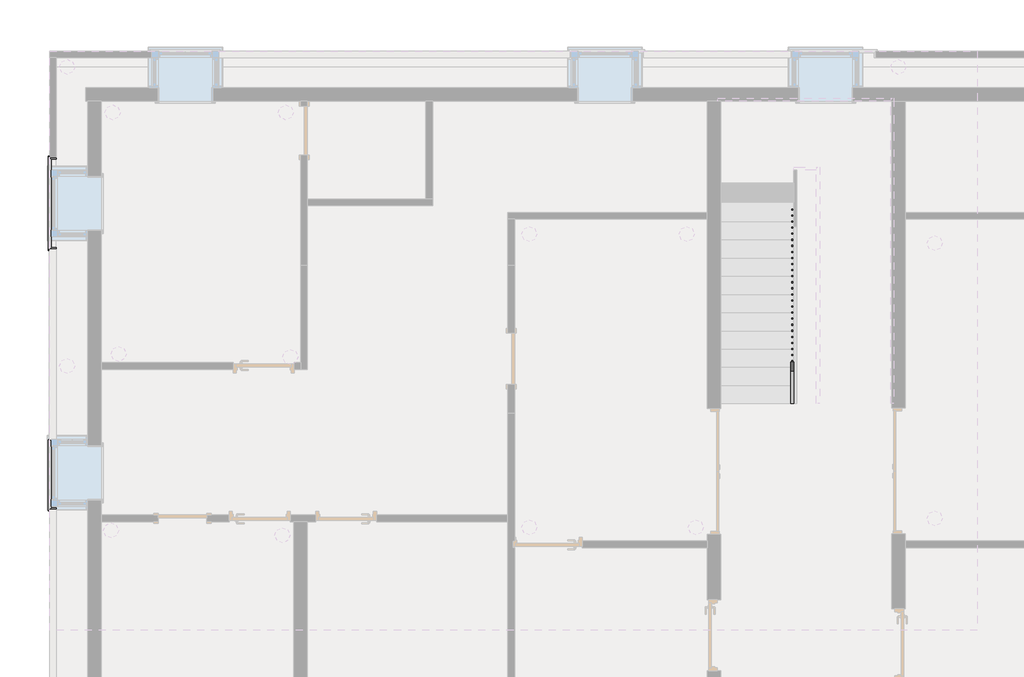
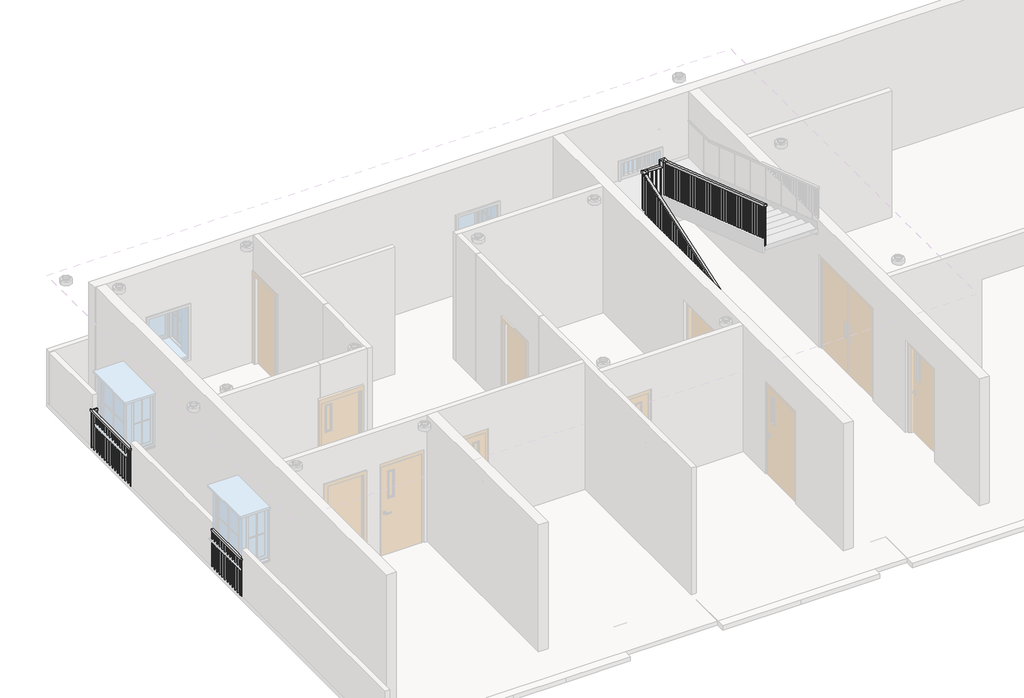
# One storey, part 4 of 7: 3 railings.
"""IFC4 building model written with IfcOpenShell, lengths in millimetres."""

from ifc_helpers import new_model, si_unit, frame, origin, place, context, project, spatial, polyline, outline, extrude, faceted_brep, element, save

model = new_model("IFC4")

# Units and contexts
model_context = context("Model", 3, world=origin())
ifc_project = project(units=[si_unit("LENGTHUNIT", "METRE", prefix="MILLI")], contexts=[model_context])

# Site, building, storey
site = spatial("IfcSite", under=ifc_project)
building = spatial("IfcBuilding", under=site)
storey = spatial("IfcBuildingStorey", under=building, Elevation=3200.4)

# Railings
placement = place(None, origin())
element("IfcRailing", 1, ObjectType="Handrail - Rectangular", at=placement, inside=storey, context=model_context, shape_type="SolidModel", body=[
    faceted_brep([(-680.3987998, 2564.5067329, 4218.2142857), (-680.3987998, 2564.5067329, 4164.5699957), (-629.5987998, 2564.5067329, 4164.5699957), (-629.5987998, 2564.5067329, 4218.2142857), (-680.3987998, 6450.7067329, 5536.7464286), (-680.3987998, 6501.5067329, 5500.3378529), (-629.5987998, 6501.5067329, 5500.3378529), (-629.5987998, 6450.7067329, 5536.7464286), (-553.3987998, 6577.7067329, 5511.8), (-553.3987998, 6577.7067329, 5562.6), (-273.9987915, 6577.7067329, 5562.6), (-223.1987915, 6577.7067329, 5511.8), (-553.3987998, 6526.9067329, 5511.8), (-223.1987915, 6526.9067329, 5511.8), (-553.3987998, 6526.9067329, 5562.6), (-273.9987915, 6526.9067329, 5562.6), (-146.9987915, 2564.5067329, 7010.4), (-197.7987915, 2564.5067329, 7010.4), (-197.7987915, 2564.5067329, 6956.75571), (-146.9987915, 2564.5067329, 6956.75571), (-146.9987915, 6442.3235624, 5641.0678571), (-146.9987915, 6450.7067329, 5691.8678571), (-197.7987915, 6442.3235624, 5641.0678571), (-197.7987915, 6450.7067329, 5691.8678571), (-680.3987998, 6450.7067329, 5562.6), (-680.3987998, 6501.5067329, 5511.8), (-629.5987998, 6501.5067329, 5511.8), (-629.5987998, 6450.7067329, 5562.6), (-680.3987998, 6577.7067329, 5562.6), (-680.3987998, 6577.7067329, 5511.8), (-629.5987998, 6526.9067329, 5511.8), (-629.5987998, 6526.9067329, 5562.6), (-273.9987915, 6577.7067329, 5691.8678571), (-223.1987915, 6577.7067329, 5641.0678571), (-223.1987915, 6526.9067329, 5641.0678571), (-273.9987915, 6526.9067329, 5691.8678571), (-146.9987915, 6577.7067329, 5691.8678571), (-146.9987915, 6577.7067329, 5641.0678571), (-197.7987915, 6526.9067329, 5641.0678571), (-197.7987915, 6526.9067329, 5691.8678571)], [[[0, 1, 2, 3]], [[1, 0, 4, 5]], [[2, 1, 5, 6]], [[3, 2, 6, 7]], [[0, 3, 7, 4]], [[8, 9, 10, 11]], [[12, 8, 11, 13]], [[14, 12, 13, 15]], [[9, 14, 15, 10]], [[16, 17, 18, 19]], [[20, 21, 16, 19]], [[22, 20, 19, 18]], [[23, 22, 18, 17]], [[21, 23, 17, 16]], [[5, 4, 24, 25]], [[6, 5, 25, 26]], [[7, 6, 26, 27]], [[4, 7, 27, 24]], [[25, 24, 28, 29]], [[26, 25, 29, 30]], [[27, 26, 30, 31]], [[24, 27, 31, 28]], [[29, 28, 9, 8]], [[30, 29, 8, 12]], [[31, 30, 12, 14]], [[28, 31, 14, 9]], [[11, 10, 32, 33]], [[13, 11, 33, 34]], [[15, 13, 34, 35]], [[10, 15, 35, 32]], [[33, 32, 36, 37]], [[34, 33, 37, 38]], [[35, 34, 38, 39]], [[32, 35, 39, 36]], [[37, 36, 21, 20]], [[38, 37, 20, 22]], [[39, 38, 22, 23]], [[36, 39, 23, 21]]]),
    extrude(outline(polyline([(2580.3817329, 6951.3695493), (2599.4317329, 6944.9061565), (2599.4317329, 5992.5857143), (2580.3817329, 5992.5857143), (2580.3817329, 6951.3695493)])), frame((-181.9237915, 0.0, 0.0), z_axis=(1.0, 0.0, 0.0), x_axis=(0.0, 1.0, 0.0)), (0.0, 0.0, 1.0), 19.05),
    extrude(outline(polyline([(2681.9817329, 6916.8981207), (2701.0317329, 6910.4347279), (2701.0317329, 5992.5857143), (2681.9817329, 5992.5857143), (2681.9817329, 6916.8981207)])), frame((-181.9237915, 0.0, 0.0), z_axis=(1.0, 0.0, 0.0), x_axis=(0.0, 1.0, 0.0)), (0.0, 0.0, 1.0), 19.05),
    extrude(outline(polyline([(2783.5817329, 6882.4266922), (2802.6317329, 6875.9632993), (2802.6317329, 5992.5857143), (2783.5817329, 5992.5857143), (2783.5817329, 6882.4266922)])), frame((-181.9237915, 0.0, 0.0), z_axis=(1.0, 0.0, 0.0), x_axis=(0.0, 1.0, 0.0)), (0.0, 0.0, 1.0), 19.05),
    extrude(outline(polyline([(2885.1817329, 6847.9552636), (2904.2317329, 6841.4918707), (2904.2317329, 5889.1714286), (2885.1817329, 5889.1714286), (2885.1817329, 6847.9552636)])), frame((-181.9237915, 0.0, 0.0), z_axis=(1.0, 0.0, 0.0), x_axis=(0.0, 1.0, 0.0)), (0.0, 0.0, 1.0), 19.05),
    extrude(outline(polyline([(2986.7817329, 6813.483835), (3005.8317329, 6807.0204422), (3005.8317329, 5889.1714286), (2986.7817329, 5889.1714286), (2986.7817329, 6813.483835)])), frame((-181.9237915, 0.0, 0.0), z_axis=(1.0, 0.0, 0.0), x_axis=(0.0, 1.0, 0.0)), (0.0, 0.0, 1.0), 19.05),
    extrude(outline(polyline([(3088.3817329, 6779.0124065), (3107.4317329, 6772.5490136), (3107.4317329, 5889.1714286), (3088.3817329, 5889.1714286), (3088.3817329, 6779.0124065)])), frame((-181.9237915, 0.0, 0.0), z_axis=(1.0, 0.0, 0.0), x_axis=(0.0, 1.0, 0.0)), (0.0, 0.0, 1.0), 19.05),
    extrude(outline(polyline([(3189.9817329, 6744.5409779), (3209.0317329, 6738.077585), (3209.0317329, 5785.7571429), (3189.9817329, 5785.7571429), (3189.9817329, 6744.5409779)])), frame((-181.9237915, 0.0, 0.0), z_axis=(1.0, 0.0, 0.0), x_axis=(0.0, 1.0, 0.0)), (0.0, 0.0, 1.0), 19.05),
    extrude(outline(polyline([(3291.5817329, 6710.0695493), (3310.6317329, 6703.6061565), (3310.6317329, 5785.7571429), (3291.5817329, 5785.7571429), (3291.5817329, 6710.0695493)])), frame((-181.9237915, 0.0, 0.0), z_axis=(1.0, 0.0, 0.0), x_axis=(0.0, 1.0, 0.0)), (0.0, 0.0, 1.0), 19.05),
    extrude(outline(polyline([(3393.1817329, 6675.5981207), (3412.2317329, 6669.1347279), (3412.2317329, 5785.7571429), (3393.1817329, 5785.7571429), (3393.1817329, 6675.5981207)])), frame((-181.9237915, 0.0, 0.0), z_axis=(1.0, 0.0, 0.0), x_axis=(0.0, 1.0, 0.0)), (0.0, 0.0, 1.0), 19.05),
    extrude(outline(polyline([(3494.7817329, 6641.1266922), (3513.8317329, 6634.6632993), (3513.8317329, 5682.3428571), (3494.7817329, 5682.3428571), (3494.7817329, 6641.1266922)])), frame((-181.9237915, 0.0, 0.0), z_axis=(1.0, 0.0, 0.0), x_axis=(0.0, 1.0, 0.0)), (0.0, 0.0, 1.0), 19.05),
    extrude(outline(polyline([(3596.3817329, 6606.6552636), (3615.4317329, 6600.1918707), (3615.4317329, 5682.3428571), (3596.3817329, 5682.3428571), (3596.3817329, 6606.6552636)])), frame((-181.9237915, 0.0, 0.0), z_axis=(1.0, 0.0, 0.0), x_axis=(0.0, 1.0, 0.0)), (0.0, 0.0, 1.0), 19.05),
    extrude(outline(polyline([(3697.9817329, 6572.183835), (3717.0317329, 6565.7204422), (3717.0317329, 5682.3428571), (3697.9817329, 5682.3428571), (3697.9817329, 6572.183835)])), frame((-181.9237915, 0.0, 0.0), z_axis=(1.0, 0.0, 0.0), x_axis=(0.0, 1.0, 0.0)), (0.0, 0.0, 1.0), 19.05),
    extrude(outline(polyline([(3799.5817329, 6537.7124065), (3818.6317329, 6531.2490136), (3818.6317329, 5578.9285714), (3799.5817329, 5578.9285714), (3799.5817329, 6537.7124065)])), frame((-181.9237915, 0.0, 0.0), z_axis=(1.0, 0.0, 0.0), x_axis=(0.0, 1.0, 0.0)), (0.0, 0.0, 1.0), 19.05),
    extrude(outline(polyline([(3901.1817329, 6503.2409779), (3920.2317329, 6496.777585), (3920.2317329, 5578.9285714), (3901.1817329, 5578.9285714), (3901.1817329, 6503.2409779)])), frame((-181.9237915, 0.0, 0.0), z_axis=(1.0, 0.0, 0.0), x_axis=(0.0, 1.0, 0.0)), (0.0, 0.0, 1.0), 19.05),
    extrude(outline(polyline([(4002.7817329, 6468.7695493), (4021.8317329, 6462.3061565), (4021.8317329, 5578.9285714), (4002.7817329, 5578.9285714), (4002.7817329, 6468.7695493)])), frame((-181.9237915, 0.0, 0.0), z_axis=(1.0, 0.0, 0.0), x_axis=(0.0, 1.0, 0.0)), (0.0, 0.0, 1.0), 19.05),
    extrude(outline(polyline([(4104.3817329, 6434.2981207), (4123.4317329, 6427.8347279), (4123.4317329, 5475.5142857), (4104.3817329, 5475.5142857), (4104.3817329, 6434.2981207)])), frame((-181.9237915, 0.0, 0.0), z_axis=(1.0, 0.0, 0.0), x_axis=(0.0, 1.0, 0.0)), (0.0, 0.0, 1.0), 19.05),
    extrude(outline(polyline([(4205.9817329, 6399.8266922), (4225.0317329, 6393.3632993), (4225.0317329, 5475.5142857), (4205.9817329, 5475.5142857), (4205.9817329, 6399.8266922)])), frame((-181.9237915, 0.0, 0.0), z_axis=(1.0, 0.0, 0.0), x_axis=(0.0, 1.0, 0.0)), (0.0, 0.0, 1.0), 19.05),
    extrude(outline(polyline([(4307.5817329, 6365.3552636), (4326.6317329, 6358.8918707), (4326.6317329, 5475.5142857), (4307.5817329, 5475.5142857), (4307.5817329, 6365.3552636)])), frame((-181.9237915, 0.0, 0.0), z_axis=(1.0, 0.0, 0.0), x_axis=(0.0, 1.0, 0.0)), (0.0, 0.0, 1.0), 19.05),
    extrude(outline(polyline([(4409.1817329, 6330.883835), (4428.2317329, 6324.4204422), (4428.2317329, 5372.1), (4409.1817329, 5372.1), (4409.1817329, 6330.883835)])), frame((-181.9237915, 0.0, 0.0), z_axis=(1.0, 0.0, 0.0), x_axis=(0.0, 1.0, 0.0)), (0.0, 0.0, 1.0), 19.05),
    extrude(outline(polyline([(4510.7817329, 6296.4124065), (4529.8317329, 6289.9490136), (4529.8317329, 5372.1), (4510.7817329, 5372.1), (4510.7817329, 6296.4124065)])), frame((-181.9237915, 0.0, 0.0), z_axis=(1.0, 0.0, 0.0), x_axis=(0.0, 1.0, 0.0)), (0.0, 0.0, 1.0), 19.05),
    extrude(outline(polyline([(4612.3817329, 6261.9409779), (4631.4317329, 6255.477585), (4631.4317329, 5372.1), (4612.3817329, 5372.1), (4612.3817329, 6261.9409779)])), frame((-181.9237915, 0.0, 0.0), z_axis=(1.0, 0.0, 0.0), x_axis=(0.0, 1.0, 0.0)), (0.0, 0.0, 1.0), 19.05),
    extrude(outline(polyline([(4713.9817329, 6227.4695493), (4733.0317329, 6221.0061565), (4733.0317329, 5268.6857143), (4713.9817329, 5268.6857143), (4713.9817329, 6227.4695493)])), frame((-181.9237915, 0.0, 0.0), z_axis=(1.0, 0.0, 0.0), x_axis=(0.0, 1.0, 0.0)), (0.0, 0.0, 1.0), 19.05),
    extrude(outline(polyline([(4815.5817329, 6192.9981207), (4834.6317329, 6186.5347279), (4834.6317329, 5268.6857143), (4815.5817329, 5268.6857143), (4815.5817329, 6192.9981207)])), frame((-181.9237915, 0.0, 0.0), z_axis=(1.0, 0.0, 0.0), x_axis=(0.0, 1.0, 0.0)), (0.0, 0.0, 1.0), 19.05),
    extrude(outline(polyline([(4917.1817329, 6158.5266922), (4936.2317329, 6152.0632993), (4936.2317329, 5268.6857143), (4917.1817329, 5268.6857143), (4917.1817329, 6158.5266922)])), frame((-181.9237915, 0.0, 0.0), z_axis=(1.0, 0.0, 0.0), x_axis=(0.0, 1.0, 0.0)), (0.0, 0.0, 1.0), 19.05),
    extrude(outline(polyline([(5018.7817329, 6124.0552636), (5037.8317329, 6117.5918707), (5037.8317329, 5165.2714286), (5018.7817329, 5165.2714286), (5018.7817329, 6124.0552636)])), frame((-181.9237915, 0.0, 0.0), z_axis=(1.0, 0.0, 0.0), x_axis=(0.0, 1.0, 0.0)), (0.0, 0.0, 1.0), 19.05),
    extrude(outline(polyline([(5120.3817329, 6089.583835), (5139.4317329, 6083.1204422), (5139.4317329, 5165.2714286), (5120.3817329, 5165.2714286), (5120.3817329, 6089.583835)])), frame((-181.9237915, 0.0, 0.0), z_axis=(1.0, 0.0, 0.0), x_axis=(0.0, 1.0, 0.0)), (0.0, 0.0, 1.0), 19.05),
    extrude(outline(polyline([(5221.9817329, 6055.1124065), (5241.0317329, 6048.6490136), (5241.0317329, 5165.2714286), (5221.9817329, 5165.2714286), (5221.9817329, 6055.1124065)])), frame((-181.9237915, 0.0, 0.0), z_axis=(1.0, 0.0, 0.0), x_axis=(0.0, 1.0, 0.0)), (0.0, 0.0, 1.0), 19.05),
    extrude(outline(polyline([(5323.5817329, 6020.6409779), (5342.6317329, 6014.177585), (5342.6317329, 5061.8571429), (5323.5817329, 5061.8571429), (5323.5817329, 6020.6409779)])), frame((-181.9237915, 0.0, 0.0), z_axis=(1.0, 0.0, 0.0), x_axis=(0.0, 1.0, 0.0)), (0.0, 0.0, 1.0), 19.05),
    extrude(outline(polyline([(5425.1817329, 5986.1695493), (5444.2317329, 5979.7061565), (5444.2317329, 5061.8571429), (5425.1817329, 5061.8571429), (5425.1817329, 5986.1695493)])), frame((-181.9237915, 0.0, 0.0), z_axis=(1.0, 0.0, 0.0), x_axis=(0.0, 1.0, 0.0)), (0.0, 0.0, 1.0), 19.05),
    extrude(outline(polyline([(5526.7817329, 5951.6981207), (5545.8317329, 5945.2347279), (5545.8317329, 5061.8571429), (5526.7817329, 5061.8571429), (5526.7817329, 5951.6981207)])), frame((-181.9237915, 0.0, 0.0), z_axis=(1.0, 0.0, 0.0), x_axis=(0.0, 1.0, 0.0)), (0.0, 0.0, 1.0), 19.05),
    extrude(outline(polyline([(5628.3817329, 5917.2266922), (5647.4317329, 5910.7632993), (5647.4317329, 4958.4428571), (5628.3817329, 4958.4428571), (5628.3817329, 5917.2266922)])), frame((-181.9237915, 0.0, 0.0), z_axis=(1.0, 0.0, 0.0), x_axis=(0.0, 1.0, 0.0)), (0.0, 0.0, 1.0), 19.05),
    extrude(outline(polyline([(5729.9817329, 5882.7552636), (5749.0317329, 5876.2918707), (5749.0317329, 4958.4428571), (5729.9817329, 4958.4428571), (5729.9817329, 5882.7552636)])), frame((-181.9237915, 0.0, 0.0), z_axis=(1.0, 0.0, 0.0), x_axis=(0.0, 1.0, 0.0)), (0.0, 0.0, 1.0), 19.05),
    extrude(outline(polyline([(5831.5817329, 5848.283835), (5850.6317329, 5841.8204422), (5850.6317329, 4958.4428571), (5831.5817329, 4958.4428571), (5831.5817329, 5848.283835)])), frame((-181.9237915, 0.0, 0.0), z_axis=(1.0, 0.0, 0.0), x_axis=(0.0, 1.0, 0.0)), (0.0, 0.0, 1.0), 19.05),
    extrude(outline(polyline([(5933.1817329, 5813.8124065), (5952.2317329, 5807.3490136), (5952.2317329, 4855.0285714), (5933.1817329, 4855.0285714), (5933.1817329, 5813.8124065)])), frame((-181.9237915, 0.0, 0.0), z_axis=(1.0, 0.0, 0.0), x_axis=(0.0, 1.0, 0.0)), (0.0, 0.0, 1.0), 19.05),
    extrude(outline(polyline([(6034.7817329, 5779.3409779), (6053.8317329, 5772.877585), (6053.8317329, 4855.0285714), (6034.7817329, 4855.0285714), (6034.7817329, 5779.3409779)])), frame((-181.9237915, 0.0, 0.0), z_axis=(1.0, 0.0, 0.0), x_axis=(0.0, 1.0, 0.0)), (0.0, 0.0, 1.0), 19.05),
    extrude(outline(polyline([(6136.3817329, 5744.8695493), (6155.4317329, 5738.4061565), (6155.4317329, 4855.0285714), (6136.3817329, 4855.0285714), (6136.3817329, 5744.8695493)])), frame((-181.9237915, 0.0, 0.0), z_axis=(1.0, 0.0, 0.0), x_axis=(0.0, 1.0, 0.0)), (0.0, 0.0, 1.0), 19.05),
    extrude(outline(polyline([(6237.9817329, 5710.3981207), (6257.0317329, 5703.9347279), (6257.0317329, 4751.6142857), (6237.9817329, 4751.6142857), (6237.9817329, 5710.3981207)])), frame((-181.9237915, 0.0, 0.0), z_axis=(1.0, 0.0, 0.0), x_axis=(0.0, 1.0, 0.0)), (0.0, 0.0, 1.0), 19.05),
    extrude(outline(polyline([(6339.5817329, 5675.9266922), (6358.6317329, 5669.4632993), (6358.6317329, 4751.6142857), (6339.5817329, 4751.6142857), (6339.5817329, 5675.9266922)])), frame((-181.9237915, 0.0, 0.0), z_axis=(1.0, 0.0, 0.0), x_axis=(0.0, 1.0, 0.0)), (0.0, 0.0, 1.0), 19.05),
    extrude(outline(polyline([(6441.1817329, 5641.4552636), (6460.2317329, 5634.9918707), (6460.2317329, 4751.6142857), (6441.1817329, 4751.6142857), (6441.1817329, 5641.4552636)])), frame((-181.9237915, 0.0, 0.0), z_axis=(1.0, 0.0, 0.0), x_axis=(0.0, 1.0, 0.0)), (0.0, 0.0, 1.0), 19.05),
    extrude(outline(polyline([(-258.1237998, 6542.7817329), (-258.1237998, 6561.8317329), (-239.0737998, 6561.8317329), (-239.0737998, 6542.7817329), (-258.1237998, 6542.7817329)])), frame((0.0, 0.0, 4648.2), z_axis=(0.0, 0.0, 1.0), x_axis=(1.0, 0.0, 0.0)), (0.0, 0.0, 1.0), 992.8678571),
    extrude(outline(polyline([(-359.7237998, 6542.7817329), (-359.7237998, 6561.8317329), (-340.6737998, 6561.8317329), (-340.6737998, 6542.7817329), (-359.7237998, 6542.7817329)])), frame((0.0, 0.0, 4648.2), z_axis=(0.0, 0.0, 1.0), x_axis=(1.0, 0.0, 0.0)), (0.0, 0.0, 1.0), 863.6),
    extrude(outline(polyline([(-461.3237998, 6542.7817329), (-461.3237998, 6561.8317329), (-442.2737998, 6561.8317329), (-442.2737998, 6542.7817329), (-461.3237998, 6542.7817329)])), frame((0.0, 0.0, 4648.2), z_axis=(0.0, 0.0, 1.0), x_axis=(1.0, 0.0, 0.0)), (0.0, 0.0, 1.0), 863.6),
    extrude(outline(polyline([(-562.9237998, 6542.7817329), (-562.9237998, 6561.8317329), (-543.8737998, 6561.8317329), (-543.8737998, 6542.7817329), (-562.9237998, 6542.7817329)])), frame((0.0, 0.0, 4648.2), z_axis=(0.0, 0.0, 1.0), x_axis=(1.0, 0.0, 0.0)), (0.0, 0.0, 1.0), 863.6),
    extrude(outline(polyline([(-645.4737998, 6517.3817329), (-664.5237998, 6517.3817329), (-664.5237998, 6536.4317329), (-645.4737998, 6536.4317329), (-645.4737998, 6517.3817329)])), frame((0.0, 0.0, 4648.2), z_axis=(0.0, 0.0, 1.0), x_axis=(1.0, 0.0, 0.0)), (0.0, 0.0, 1.0), 863.6),
    extrude(outline(polyline([(6415.7817329, 5471.252585), (6434.8317329, 5477.7159779), (6434.8317329, 4544.7857143), (6415.7817329, 4544.7857143), (6415.7817329, 5471.252585)])), frame((-664.5237998, 0.0, 0.0), z_axis=(1.0, 0.0, 0.0), x_axis=(0.0, 1.0, 0.0)), (0.0, 0.0, 1.0), 19.05),
    extrude(outline(polyline([(6314.1817329, 5436.7811565), (6333.2317329, 5443.2445493), (6333.2317329, 4544.7857143), (6314.1817329, 4544.7857143), (6314.1817329, 5436.7811565)])), frame((-664.5237998, 0.0, 0.0), z_axis=(1.0, 0.0, 0.0), x_axis=(0.0, 1.0, 0.0)), (0.0, 0.0, 1.0), 19.05),
    extrude(outline(polyline([(6212.5817329, 5402.3097279), (6231.6317329, 5408.7731207), (6231.6317329, 4544.7857143), (6212.5817329, 4544.7857143), (6212.5817329, 5402.3097279)])), frame((-664.5237998, 0.0, 0.0), z_axis=(1.0, 0.0, 0.0), x_axis=(0.0, 1.0, 0.0)), (0.0, 0.0, 1.0), 19.05),
    extrude(outline(polyline([(6110.9817329, 5367.8382993), (6130.0317329, 5374.3016922), (6130.0317329, 4441.3714286), (6110.9817329, 4441.3714286), (6110.9817329, 5367.8382993)])), frame((-664.5237998, 0.0, 0.0), z_axis=(1.0, 0.0, 0.0), x_axis=(0.0, 1.0, 0.0)), (0.0, 0.0, 1.0), 19.05),
    extrude(outline(polyline([(6009.3817329, 5333.3668707), (6028.4317329, 5339.8302636), (6028.4317329, 4441.3714286), (6009.3817329, 4441.3714286), (6009.3817329, 5333.3668707)])), frame((-664.5237998, 0.0, 0.0), z_axis=(1.0, 0.0, 0.0), x_axis=(0.0, 1.0, 0.0)), (0.0, 0.0, 1.0), 19.05),
    extrude(outline(polyline([(5907.7817329, 5298.8954422), (5926.8317329, 5305.358835), (5926.8317329, 4441.3714286), (5907.7817329, 4441.3714286), (5907.7817329, 5298.8954422)])), frame((-664.5237998, 0.0, 0.0), z_axis=(1.0, 0.0, 0.0), x_axis=(0.0, 1.0, 0.0)), (0.0, 0.0, 1.0), 19.05),
    extrude(outline(polyline([(5806.1817329, 5264.4240136), (5825.2317329, 5270.8874065), (5825.2317329, 4337.9571429), (5806.1817329, 4337.9571429), (5806.1817329, 5264.4240136)])), frame((-664.5237998, 0.0, 0.0), z_axis=(1.0, 0.0, 0.0), x_axis=(0.0, 1.0, 0.0)), (0.0, 0.0, 1.0), 19.05),
    extrude(outline(polyline([(5704.5817329, 5229.952585), (5723.6317329, 5236.4159779), (5723.6317329, 4337.9571429), (5704.5817329, 4337.9571429), (5704.5817329, 5229.952585)])), frame((-664.5237998, 0.0, 0.0), z_axis=(1.0, 0.0, 0.0), x_axis=(0.0, 1.0, 0.0)), (0.0, 0.0, 1.0), 19.05),
    extrude(outline(polyline([(5602.9817329, 5195.4811565), (5622.0317329, 5201.9445493), (5622.0317329, 4337.9571429), (5602.9817329, 4337.9571429), (5602.9817329, 5195.4811565)])), frame((-664.5237998, 0.0, 0.0), z_axis=(1.0, 0.0, 0.0), x_axis=(0.0, 1.0, 0.0)), (0.0, 0.0, 1.0), 19.05),
    extrude(outline(polyline([(5501.3817329, 5161.0097279), (5520.4317329, 5167.4731207), (5520.4317329, 4234.5428571), (5501.3817329, 4234.5428571), (5501.3817329, 5161.0097279)])), frame((-664.5237998, 0.0, 0.0), z_axis=(1.0, 0.0, 0.0), x_axis=(0.0, 1.0, 0.0)), (0.0, 0.0, 1.0), 19.05),
    extrude(outline(polyline([(5399.7817329, 5126.5382993), (5418.8317329, 5133.0016922), (5418.8317329, 4234.5428571), (5399.7817329, 4234.5428571), (5399.7817329, 5126.5382993)])), frame((-664.5237998, 0.0, 0.0), z_axis=(1.0, 0.0, 0.0), x_axis=(0.0, 1.0, 0.0)), (0.0, 0.0, 1.0), 19.05),
    extrude(outline(polyline([(5298.1817329, 5092.0668707), (5317.2317329, 5098.5302636), (5317.2317329, 4234.5428571), (5298.1817329, 4234.5428571), (5298.1817329, 5092.0668707)])), frame((-664.5237998, 0.0, 0.0), z_axis=(1.0, 0.0, 0.0), x_axis=(0.0, 1.0, 0.0)), (0.0, 0.0, 1.0), 19.05),
    extrude(outline(polyline([(5196.5817329, 5057.5954422), (5215.6317329, 5064.058835), (5215.6317329, 4131.1285714), (5196.5817329, 4131.1285714), (5196.5817329, 5057.5954422)])), frame((-664.5237998, 0.0, 0.0), z_axis=(1.0, 0.0, 0.0), x_axis=(0.0, 1.0, 0.0)), (0.0, 0.0, 1.0), 19.05),
    extrude(outline(polyline([(5094.9817329, 5023.1240136), (5114.0317329, 5029.5874065), (5114.0317329, 4131.1285714), (5094.9817329, 4131.1285714), (5094.9817329, 5023.1240136)])), frame((-664.5237998, 0.0, 0.0), z_axis=(1.0, 0.0, 0.0), x_axis=(0.0, 1.0, 0.0)), (0.0, 0.0, 1.0), 19.05),
    extrude(outline(polyline([(4993.3817329, 4988.652585), (5012.4317329, 4995.1159779), (5012.4317329, 4131.1285714), (4993.3817329, 4131.1285714), (4993.3817329, 4988.652585)])), frame((-664.5237998, 0.0, 0.0), z_axis=(1.0, 0.0, 0.0), x_axis=(0.0, 1.0, 0.0)), (0.0, 0.0, 1.0), 19.05),
    extrude(outline(polyline([(4891.7817329, 4954.1811565), (4910.8317329, 4960.6445493), (4910.8317329, 4027.7142857), (4891.7817329, 4027.7142857), (4891.7817329, 4954.1811565)])), frame((-664.5237998, 0.0, 0.0), z_axis=(1.0, 0.0, 0.0), x_axis=(0.0, 1.0, 0.0)), (0.0, 0.0, 1.0), 19.05),
    extrude(outline(polyline([(4790.1817329, 4919.7097279), (4809.2317329, 4926.1731207), (4809.2317329, 4027.7142857), (4790.1817329, 4027.7142857), (4790.1817329, 4919.7097279)])), frame((-664.5237998, 0.0, 0.0), z_axis=(1.0, 0.0, 0.0), x_axis=(0.0, 1.0, 0.0)), (0.0, 0.0, 1.0), 19.05),
    extrude(outline(polyline([(4688.5817329, 4885.2382993), (4707.6317329, 4891.7016922), (4707.6317329, 4027.7142857), (4688.5817329, 4027.7142857), (4688.5817329, 4885.2382993)])), frame((-664.5237998, 0.0, 0.0), z_axis=(1.0, 0.0, 0.0), x_axis=(0.0, 1.0, 0.0)), (0.0, 0.0, 1.0), 19.05),
    extrude(outline(polyline([(4586.9817329, 4850.7668707), (4606.0317329, 4857.2302636), (4606.0317329, 3924.3), (4586.9817329, 3924.3), (4586.9817329, 4850.7668707)])), frame((-664.5237998, 0.0, 0.0), z_axis=(1.0, 0.0, 0.0), x_axis=(0.0, 1.0, 0.0)), (0.0, 0.0, 1.0), 19.05),
    extrude(outline(polyline([(4485.3817329, 4816.2954422), (4504.4317329, 4822.758835), (4504.4317329, 3924.3), (4485.3817329, 3924.3), (4485.3817329, 4816.2954422)])), frame((-664.5237998, 0.0, 0.0), z_axis=(1.0, 0.0, 0.0), x_axis=(0.0, 1.0, 0.0)), (0.0, 0.0, 1.0), 19.05),
    extrude(outline(polyline([(4383.7817329, 4781.8240136), (4402.8317329, 4788.2874065), (4402.8317329, 3924.3), (4383.7817329, 3924.3), (4383.7817329, 4781.8240136)])), frame((-664.5237998, 0.0, 0.0), z_axis=(1.0, 0.0, 0.0), x_axis=(0.0, 1.0, 0.0)), (0.0, 0.0, 1.0), 19.05),
    extrude(outline(polyline([(4282.1817329, 4747.352585), (4301.2317329, 4753.8159779), (4301.2317329, 3820.8857143), (4282.1817329, 3820.8857143), (4282.1817329, 4747.352585)])), frame((-664.5237998, 0.0, 0.0), z_axis=(1.0, 0.0, 0.0), x_axis=(0.0, 1.0, 0.0)), (0.0, 0.0, 1.0), 19.05),
    extrude(outline(polyline([(4180.5817329, 4712.8811565), (4199.6317329, 4719.3445493), (4199.6317329, 3820.8857143), (4180.5817329, 3820.8857143), (4180.5817329, 4712.8811565)])), frame((-664.5237998, 0.0, 0.0), z_axis=(1.0, 0.0, 0.0), x_axis=(0.0, 1.0, 0.0)), (0.0, 0.0, 1.0), 19.05),
    extrude(outline(polyline([(4078.9817329, 4678.4097279), (4098.0317329, 4684.8731207), (4098.0317329, 3820.8857143), (4078.9817329, 3820.8857143), (4078.9817329, 4678.4097279)])), frame((-664.5237998, 0.0, 0.0), z_axis=(1.0, 0.0, 0.0), x_axis=(0.0, 1.0, 0.0)), (0.0, 0.0, 1.0), 19.05),
    extrude(outline(polyline([(3977.3817329, 4643.9382993), (3996.4317329, 4650.4016922), (3996.4317329, 3717.4714286), (3977.3817329, 3717.4714286), (3977.3817329, 4643.9382993)])), frame((-664.5237998, 0.0, 0.0), z_axis=(1.0, 0.0, 0.0), x_axis=(0.0, 1.0, 0.0)), (0.0, 0.0, 1.0), 19.05),
    extrude(outline(polyline([(3875.7817329, 4609.4668707), (3894.8317329, 4615.9302636), (3894.8317329, 3717.4714286), (3875.7817329, 3717.4714286), (3875.7817329, 4609.4668707)])), frame((-664.5237998, 0.0, 0.0), z_axis=(1.0, 0.0, 0.0), x_axis=(0.0, 1.0, 0.0)), (0.0, 0.0, 1.0), 19.05),
    extrude(outline(polyline([(3774.1817329, 4574.9954422), (3793.2317329, 4581.458835), (3793.2317329, 3717.4714286), (3774.1817329, 3717.4714286), (3774.1817329, 4574.9954422)])), frame((-664.5237998, 0.0, 0.0), z_axis=(1.0, 0.0, 0.0), x_axis=(0.0, 1.0, 0.0)), (0.0, 0.0, 1.0), 19.05),
    extrude(outline(polyline([(3672.5817329, 4540.5240136), (3691.6317329, 4546.9874065), (3691.6317329, 3614.0571429), (3672.5817329, 3614.0571429), (3672.5817329, 4540.5240136)])), frame((-664.5237998, 0.0, 0.0), z_axis=(1.0, 0.0, 0.0), x_axis=(0.0, 1.0, 0.0)), (0.0, 0.0, 1.0), 19.05),
    extrude(outline(polyline([(3570.9817329, 4506.052585), (3590.0317329, 4512.5159779), (3590.0317329, 3614.0571429), (3570.9817329, 3614.0571429), (3570.9817329, 4506.052585)])), frame((-664.5237998, 0.0, 0.0), z_axis=(1.0, 0.0, 0.0), x_axis=(0.0, 1.0, 0.0)), (0.0, 0.0, 1.0), 19.05),
    extrude(outline(polyline([(3469.3817329, 4471.5811565), (3488.4317329, 4478.0445493), (3488.4317329, 3614.0571429), (3469.3817329, 3614.0571429), (3469.3817329, 4471.5811565)])), frame((-664.5237998, 0.0, 0.0), z_axis=(1.0, 0.0, 0.0), x_axis=(0.0, 1.0, 0.0)), (0.0, 0.0, 1.0), 19.05),
    extrude(outline(polyline([(3367.7817329, 4437.1097279), (3386.8317329, 4443.5731207), (3386.8317329, 3510.6428571), (3367.7817329, 3510.6428571), (3367.7817329, 4437.1097279)])), frame((-664.5237998, 0.0, 0.0), z_axis=(1.0, 0.0, 0.0), x_axis=(0.0, 1.0, 0.0)), (0.0, 0.0, 1.0), 19.05),
    extrude(outline(polyline([(3266.1817329, 4402.6382993), (3285.2317329, 4409.1016922), (3285.2317329, 3510.6428571), (3266.1817329, 3510.6428571), (3266.1817329, 4402.6382993)])), frame((-664.5237998, 0.0, 0.0), z_axis=(1.0, 0.0, 0.0), x_axis=(0.0, 1.0, 0.0)), (0.0, 0.0, 1.0), 19.05),
    extrude(outline(polyline([(3164.5817329, 4368.1668707), (3183.6317329, 4374.6302636), (3183.6317329, 3510.6428571), (3164.5817329, 3510.6428571), (3164.5817329, 4368.1668707)])), frame((-664.5237998, 0.0, 0.0), z_axis=(1.0, 0.0, 0.0), x_axis=(0.0, 1.0, 0.0)), (0.0, 0.0, 1.0), 19.05),
    extrude(outline(polyline([(3062.9817329, 4333.6954422), (3082.0317329, 4340.158835), (3082.0317329, 3407.2285714), (3062.9817329, 3407.2285714), (3062.9817329, 4333.6954422)])), frame((-664.5237998, 0.0, 0.0), z_axis=(1.0, 0.0, 0.0), x_axis=(0.0, 1.0, 0.0)), (0.0, 0.0, 1.0), 19.05),
    extrude(outline(polyline([(2961.3817329, 4299.2240136), (2980.4317329, 4305.6874065), (2980.4317329, 3407.2285714), (2961.3817329, 3407.2285714), (2961.3817329, 4299.2240136)])), frame((-664.5237998, 0.0, 0.0), z_axis=(1.0, 0.0, 0.0), x_axis=(0.0, 1.0, 0.0)), (0.0, 0.0, 1.0), 19.05),
    extrude(outline(polyline([(2859.7817329, 4264.752585), (2878.8317329, 4271.2159779), (2878.8317329, 3407.2285714), (2859.7817329, 3407.2285714), (2859.7817329, 4264.752585)])), frame((-664.5237998, 0.0, 0.0), z_axis=(1.0, 0.0, 0.0), x_axis=(0.0, 1.0, 0.0)), (0.0, 0.0, 1.0), 19.05),
    extrude(outline(polyline([(2758.1817329, 4230.2811565), (2777.2317329, 4236.7445493), (2777.2317329, 3303.8142857), (2758.1817329, 3303.8142857), (2758.1817329, 4230.2811565)])), frame((-664.5237998, 0.0, 0.0), z_axis=(1.0, 0.0, 0.0), x_axis=(0.0, 1.0, 0.0)), (0.0, 0.0, 1.0), 19.05),
    extrude(outline(polyline([(2656.5817329, 4195.8097279), (2675.6317329, 4202.2731207), (2675.6317329, 3303.8142857), (2656.5817329, 3303.8142857), (2656.5817329, 4195.8097279)])), frame((-664.5237998, 0.0, 0.0), z_axis=(1.0, 0.0, 0.0), x_axis=(0.0, 1.0, 0.0)), (0.0, 0.0, 1.0), 19.05),
    extrude(outline(polyline([(-181.9237915, 6542.7817329), (-181.9237915, 6561.8317329), (-162.8737915, 6561.8317329), (-162.8737915, 6542.7817329), (-181.9237915, 6542.7817329)])), frame((0.0, 0.0, 4648.2), z_axis=(0.0, 0.0, 1.0), x_axis=(1.0, 0.0, 0.0)), (0.0, 0.0, 1.0), 992.8678571),
    extrude(outline(polyline([(-645.4737998, 6542.7817329), (-664.5237998, 6542.7817329), (-664.5237998, 6561.8317329), (-645.4737998, 6561.8317329), (-645.4737998, 6542.7817329)])), frame((0.0, 0.0, 4648.2), z_axis=(0.0, 0.0, 1.0), x_axis=(1.0, 0.0, 0.0)), (0.0, 0.0, 1.0), 863.6),
    extrude(outline(polyline([(2564.5067329, 6956.75571), (2583.5567329, 6950.2923172), (2583.5567329, 5992.5857143), (2564.5067329, 5992.5857143), (2564.5067329, 6956.75571)])), frame((-181.9237915, 0.0, 0.0), z_axis=(1.0, 0.0, 0.0), x_axis=(0.0, 1.0, 0.0)), (0.0, 0.0, 1.0), 19.05),
    extrude(outline(polyline([(2564.5067329, 4164.5699957), (2583.5567329, 4171.0333886), (2583.5567329, 3303.8142857), (2564.5067329, 3303.8142857), (2564.5067329, 4164.5699957)])), frame((-664.5237998, 0.0, 0.0), z_axis=(1.0, 0.0, 0.0), x_axis=(0.0, 1.0, 0.0)), (0.0, 0.0, 1.0), 19.05),
])
element("IfcRailing", 2, ObjectType="Handrail - Rectangular", at=placement, inside=storey, context=model_context, shape_type="SolidModel", body=[
    faceted_brep([(-13063.4067989, 1953.9604213, 4114.8), (-13063.4067989, 1953.9604213, 4064.0), (-13114.2067989, 1953.9604213, 4064.0), (-13114.2067989, 1953.9604213, 4114.8), (-13063.4067989, 818.2567339, 4114.8), (-13063.4067989, 818.2567339, 4064.0), (-13114.2067989, 767.4567339, 4064.0), (-13114.2067989, 767.4567339, 4114.8), (-12974.5067989, 818.2567339, 4114.8), (-12974.5067989, 767.4567339, 4114.8), (-12974.5067989, 767.4567339, 4064.0), (-12974.5067989, 818.2567339, 4064.0)], [[[0, 1, 2, 3]], [[1, 0, 4, 5]], [[2, 1, 5, 6]], [[3, 2, 6, 7]], [[0, 3, 7, 4]], [[8, 9, 10, 11]], [[5, 4, 8, 11]], [[6, 5, 11, 10]], [[7, 6, 10, 9]], [[4, 7, 9, 8]]]),
    extrude(outline(polyline([(-12996.7317989, 783.3317339), (-12996.7317989, 802.3817339), (-12977.6817989, 802.3817339), (-12977.6817989, 783.3317339), (-12996.7317989, 783.3317339)])), frame((0.0, 0.0, 3200.4), z_axis=(0.0, 0.0, 1.0), x_axis=(1.0, 0.0, 0.0)), (0.0, 0.0, 1.0), 863.6),
    extrude(outline(polyline([(-13098.3317989, 845.8854213), (-13079.2817989, 845.8854213), (-13079.2817989, 826.8354213), (-13098.3317989, 826.8354213), (-13098.3317989, 845.8854213)])), frame((0.0, 0.0, 3200.4), z_axis=(0.0, 0.0, 1.0), x_axis=(1.0, 0.0, 0.0)), (0.0, 0.0, 1.0), 863.6),
    extrude(outline(polyline([(-13098.3317989, 947.4854213), (-13079.2817989, 947.4854213), (-13079.2817989, 928.4354213), (-13098.3317989, 928.4354213), (-13098.3317989, 947.4854213)])), frame((0.0, 0.0, 3200.4), z_axis=(0.0, 0.0, 1.0), x_axis=(1.0, 0.0, 0.0)), (0.0, 0.0, 1.0), 863.6),
    extrude(outline(polyline([(-13098.3317989, 1049.0854213), (-13079.2817989, 1049.0854213), (-13079.2817989, 1030.0354213), (-13098.3317989, 1030.0354213), (-13098.3317989, 1049.0854213)])), frame((0.0, 0.0, 3200.4), z_axis=(0.0, 0.0, 1.0), x_axis=(1.0, 0.0, 0.0)), (0.0, 0.0, 1.0), 863.6),
    extrude(outline(polyline([(-13098.3317989, 1150.6854213), (-13079.2817989, 1150.6854213), (-13079.2817989, 1131.6354213), (-13098.3317989, 1131.6354213), (-13098.3317989, 1150.6854213)])), frame((0.0, 0.0, 3200.4), z_axis=(0.0, 0.0, 1.0), x_axis=(1.0, 0.0, 0.0)), (0.0, 0.0, 1.0), 863.6),
    extrude(outline(polyline([(-13098.3317989, 1252.2854213), (-13079.2817989, 1252.2854213), (-13079.2817989, 1233.2354213), (-13098.3317989, 1233.2354213), (-13098.3317989, 1252.2854213)])), frame((0.0, 0.0, 3200.4), z_axis=(0.0, 0.0, 1.0), x_axis=(1.0, 0.0, 0.0)), (0.0, 0.0, 1.0), 863.6),
    extrude(outline(polyline([(-13098.3317989, 1353.8854213), (-13079.2817989, 1353.8854213), (-13079.2817989, 1334.8354213), (-13098.3317989, 1334.8354213), (-13098.3317989, 1353.8854213)])), frame((0.0, 0.0, 3200.4), z_axis=(0.0, 0.0, 1.0), x_axis=(1.0, 0.0, 0.0)), (0.0, 0.0, 1.0), 863.6),
    extrude(outline(polyline([(-13098.3317989, 1455.4854213), (-13079.2817989, 1455.4854213), (-13079.2817989, 1436.4354213), (-13098.3317989, 1436.4354213), (-13098.3317989, 1455.4854213)])), frame((0.0, 0.0, 3200.4), z_axis=(0.0, 0.0, 1.0), x_axis=(1.0, 0.0, 0.0)), (0.0, 0.0, 1.0), 863.6),
    extrude(outline(polyline([(-13098.3317989, 1557.0854213), (-13079.2817989, 1557.0854213), (-13079.2817989, 1538.0354213), (-13098.3317989, 1538.0354213), (-13098.3317989, 1557.0854213)])), frame((0.0, 0.0, 3200.4), z_axis=(0.0, 0.0, 1.0), x_axis=(1.0, 0.0, 0.0)), (0.0, 0.0, 1.0), 863.6),
    extrude(outline(polyline([(-13098.3317989, 1658.6854213), (-13079.2817989, 1658.6854213), (-13079.2817989, 1639.6354213), (-13098.3317989, 1639.6354213), (-13098.3317989, 1658.6854213)])), frame((0.0, 0.0, 3200.4), z_axis=(0.0, 0.0, 1.0), x_axis=(1.0, 0.0, 0.0)), (0.0, 0.0, 1.0), 863.6),
    extrude(outline(polyline([(-13098.3317989, 1760.2854213), (-13079.2817989, 1760.2854213), (-13079.2817989, 1741.2354213), (-13098.3317989, 1741.2354213), (-13098.3317989, 1760.2854213)])), frame((0.0, 0.0, 3200.4), z_axis=(0.0, 0.0, 1.0), x_axis=(1.0, 0.0, 0.0)), (0.0, 0.0, 1.0), 863.6),
    extrude(outline(polyline([(-13098.3317989, 1861.8854213), (-13079.2817989, 1861.8854213), (-13079.2817989, 1842.8354213), (-13098.3317989, 1842.8354213), (-13098.3317989, 1861.8854213)])), frame((0.0, 0.0, 3200.4), z_axis=(0.0, 0.0, 1.0), x_axis=(1.0, 0.0, 0.0)), (0.0, 0.0, 1.0), 863.6),
    extrude(outline(polyline([(-13098.3317989, 802.3817339), (-13079.2817989, 802.3817339), (-13079.2817989, 783.3317339), (-13098.3317989, 783.3317339), (-13098.3317989, 802.3817339)])), frame((0.0, 0.0, 3200.4), z_axis=(0.0, 0.0, 1.0), x_axis=(1.0, 0.0, 0.0)), (0.0, 0.0, 1.0), 863.6),
    extrude(outline(polyline([(-13079.2817989, 1963.4854213), (-13079.2817989, 1944.4354213), (-13098.3317989, 1944.4354213), (-13098.3317989, 1963.4854213), (-13079.2817989, 1963.4854213)])), frame((0.0, 0.0, 3200.4), z_axis=(0.0, 0.0, 1.0), x_axis=(1.0, 0.0, 0.0)), (0.0, 0.0, 1.0), 863.6),
    extrude(outline(polyline([(-12993.5567989, 783.3317339), (-12993.5567989, 802.3817339), (-12974.5067989, 802.3817339), (-12974.5067989, 783.3317339), (-12993.5567989, 783.3317339)])), frame((0.0, 0.0, 3200.4), z_axis=(0.0, 0.0, 1.0), x_axis=(1.0, 0.0, 0.0)), (0.0, 0.0, 1.0), 863.6),
    extrude(outline(polyline([(-13062.8987925, 1963.4854213), (-13062.8987925, 1944.4354213), (-13081.9487925, 1944.4354213), (-13081.9487925, 1963.4854213), (-13062.8987925, 1963.4854213)])), frame((0.0, 0.0, 3200.4), z_axis=(0.0, 0.0, 1.0), x_axis=(1.0, 0.0, 0.0)), (0.0, 0.0, 1.0), 863.6),
])
element("IfcRailing", 3, ObjectType="Handrail - Rectangular", at=placement, inside=storey, context=model_context, shape_type="SolidModel", body=[
    faceted_brep([(-12973.9987925, 6656.8711337, 4114.8), (-12973.9987925, 6656.8711337, 4064.0), (-12973.9987925, 6707.6711337, 4064.0), (-12973.9987925, 6707.6711337, 4114.8), (-13062.8987925, 6656.8711337, 4114.8), (-13062.8987925, 6656.8711337, 4064.0), (-13113.6987925, 6707.6711337, 4064.0), (-13113.6987925, 6707.6711337, 4114.8), (-13062.8987925, 5180.1736362, 4114.8), (-13062.8987925, 5180.1736362, 4064.0), (-13113.6987925, 5129.3736362, 4064.0), (-13113.6987925, 5129.3736362, 4114.8), (-12973.9987925, 5180.1736362, 4114.8), (-12973.9987925, 5129.3736362, 4114.8), (-12973.9987925, 5129.3736362, 4064.0), (-12973.9987925, 5180.1736362, 4064.0)], [[[0, 1, 2, 3]], [[1, 0, 4, 5]], [[2, 1, 5, 6]], [[3, 2, 6, 7]], [[0, 3, 7, 4]], [[5, 4, 8, 9]], [[6, 5, 9, 10]], [[7, 6, 10, 11]], [[4, 7, 11, 8]], [[12, 13, 14, 15]], [[9, 8, 12, 15]], [[10, 9, 15, 14]], [[11, 10, 14, 13]], [[8, 11, 13, 12]]]),
    extrude(outline(polyline([(-12996.2237925, 5145.2486362), (-12996.2237925, 5164.2986362), (-12977.1737925, 5164.2986362), (-12977.1737925, 5145.2486362), (-12996.2237925, 5145.2486362)])), frame((0.0, 0.0, 3200.4), z_axis=(0.0, 0.0, 1.0), x_axis=(1.0, 0.0, 0.0)), (0.0, 0.0, 1.0), 863.6),
    extrude(outline(polyline([(-13097.8237925, 5167.7961337), (-13078.7737925, 5167.7961337), (-13078.7737925, 5148.7461337), (-13097.8237925, 5148.7461337), (-13097.8237925, 5167.7961337)])), frame((0.0, 0.0, 3200.4), z_axis=(0.0, 0.0, 1.0), x_axis=(1.0, 0.0, 0.0)), (0.0, 0.0, 1.0), 863.6),
    extrude(outline(polyline([(-13097.8237925, 5269.3961337), (-13078.7737925, 5269.3961337), (-13078.7737925, 5250.3461337), (-13097.8237925, 5250.3461337), (-13097.8237925, 5269.3961337)])), frame((0.0, 0.0, 3200.4), z_axis=(0.0, 0.0, 1.0), x_axis=(1.0, 0.0, 0.0)), (0.0, 0.0, 1.0), 863.6),
    extrude(outline(polyline([(-13097.8237925, 5370.9961337), (-13078.7737925, 5370.9961337), (-13078.7737925, 5351.9461337), (-13097.8237925, 5351.9461337), (-13097.8237925, 5370.9961337)])), frame((0.0, 0.0, 3200.4), z_axis=(0.0, 0.0, 1.0), x_axis=(1.0, 0.0, 0.0)), (0.0, 0.0, 1.0), 863.6),
    extrude(outline(polyline([(-13097.8237925, 5472.5961337), (-13078.7737925, 5472.5961337), (-13078.7737925, 5453.5461337), (-13097.8237925, 5453.5461337), (-13097.8237925, 5472.5961337)])), frame((0.0, 0.0, 3200.4), z_axis=(0.0, 0.0, 1.0), x_axis=(1.0, 0.0, 0.0)), (0.0, 0.0, 1.0), 863.6),
    extrude(outline(polyline([(-13097.8237925, 5574.1961337), (-13078.7737925, 5574.1961337), (-13078.7737925, 5555.1461337), (-13097.8237925, 5555.1461337), (-13097.8237925, 5574.1961337)])), frame((0.0, 0.0, 3200.4), z_axis=(0.0, 0.0, 1.0), x_axis=(1.0, 0.0, 0.0)), (0.0, 0.0, 1.0), 863.6),
    extrude(outline(polyline([(-13097.8237925, 5675.7961337), (-13078.7737925, 5675.7961337), (-13078.7737925, 5656.7461337), (-13097.8237925, 5656.7461337), (-13097.8237925, 5675.7961337)])), frame((0.0, 0.0, 3200.4), z_axis=(0.0, 0.0, 1.0), x_axis=(1.0, 0.0, 0.0)), (0.0, 0.0, 1.0), 863.6),
    extrude(outline(polyline([(-13097.8237925, 5777.3961337), (-13078.7737925, 5777.3961337), (-13078.7737925, 5758.3461337), (-13097.8237925, 5758.3461337), (-13097.8237925, 5777.3961337)])), frame((0.0, 0.0, 3200.4), z_axis=(0.0, 0.0, 1.0), x_axis=(1.0, 0.0, 0.0)), (0.0, 0.0, 1.0), 863.6),
    extrude(outline(polyline([(-13097.8237925, 5878.9961337), (-13078.7737925, 5878.9961337), (-13078.7737925, 5859.9461337), (-13097.8237925, 5859.9461337), (-13097.8237925, 5878.9961337)])), frame((0.0, 0.0, 3200.4), z_axis=(0.0, 0.0, 1.0), x_axis=(1.0, 0.0, 0.0)), (0.0, 0.0, 1.0), 863.6),
    extrude(outline(polyline([(-13097.8237925, 5980.5961337), (-13078.7737925, 5980.5961337), (-13078.7737925, 5961.5461337), (-13097.8237925, 5961.5461337), (-13097.8237925, 5980.5961337)])), frame((0.0, 0.0, 3200.4), z_axis=(0.0, 0.0, 1.0), x_axis=(1.0, 0.0, 0.0)), (0.0, 0.0, 1.0), 863.6),
    extrude(outline(polyline([(-13097.8237925, 6082.1961337), (-13078.7737925, 6082.1961337), (-13078.7737925, 6063.1461337), (-13097.8237925, 6063.1461337), (-13097.8237925, 6082.1961337)])), frame((0.0, 0.0, 3200.4), z_axis=(0.0, 0.0, 1.0), x_axis=(1.0, 0.0, 0.0)), (0.0, 0.0, 1.0), 863.6),
    extrude(outline(polyline([(-13097.8237925, 6183.7961337), (-13078.7737925, 6183.7961337), (-13078.7737925, 6164.7461337), (-13097.8237925, 6164.7461337), (-13097.8237925, 6183.7961337)])), frame((0.0, 0.0, 3200.4), z_axis=(0.0, 0.0, 1.0), x_axis=(1.0, 0.0, 0.0)), (0.0, 0.0, 1.0), 863.6),
    extrude(outline(polyline([(-13097.8237925, 6285.3961337), (-13078.7737925, 6285.3961337), (-13078.7737925, 6266.3461337), (-13097.8237925, 6266.3461337), (-13097.8237925, 6285.3961337)])), frame((0.0, 0.0, 3200.4), z_axis=(0.0, 0.0, 1.0), x_axis=(1.0, 0.0, 0.0)), (0.0, 0.0, 1.0), 863.6),
    extrude(outline(polyline([(-13097.8237925, 6386.9961337), (-13078.7737925, 6386.9961337), (-13078.7737925, 6367.9461337), (-13097.8237925, 6367.9461337), (-13097.8237925, 6386.9961337)])), frame((0.0, 0.0, 3200.4), z_axis=(0.0, 0.0, 1.0), x_axis=(1.0, 0.0, 0.0)), (0.0, 0.0, 1.0), 863.6),
    extrude(outline(polyline([(-13097.8237925, 6488.5961337), (-13078.7737925, 6488.5961337), (-13078.7737925, 6469.5461337), (-13097.8237925, 6469.5461337), (-13097.8237925, 6488.5961337)])), frame((0.0, 0.0, 3200.4), z_axis=(0.0, 0.0, 1.0), x_axis=(1.0, 0.0, 0.0)), (0.0, 0.0, 1.0), 863.6),
    extrude(outline(polyline([(-13097.8237925, 6590.1961337), (-13078.7737925, 6590.1961337), (-13078.7737925, 6571.1461337), (-13097.8237925, 6571.1461337), (-13097.8237925, 6590.1961337)])), frame((0.0, 0.0, 3200.4), z_axis=(0.0, 0.0, 1.0), x_axis=(1.0, 0.0, 0.0)), (0.0, 0.0, 1.0), 863.6),
    extrude(outline(polyline([(-13066.0737925, 6691.7961337), (-13066.0737925, 6672.7461337), (-13085.1237925, 6672.7461337), (-13085.1237925, 6691.7961337), (-13066.0737925, 6691.7961337)])), frame((0.0, 0.0, 3200.4), z_axis=(0.0, 0.0, 1.0), x_axis=(1.0, 0.0, 0.0)), (0.0, 0.0, 1.0), 863.6),
    extrude(outline(polyline([(-13097.8237925, 5164.2986362), (-13078.7737925, 5164.2986362), (-13078.7737925, 5145.2486362), (-13097.8237925, 5145.2486362), (-13097.8237925, 5164.2986362)])), frame((0.0, 0.0, 3200.4), z_axis=(0.0, 0.0, 1.0), x_axis=(1.0, 0.0, 0.0)), (0.0, 0.0, 1.0), 863.6),
    extrude(outline(polyline([(-13078.7737925, 6691.7961337), (-13078.7737925, 6672.7461337), (-13097.8237925, 6672.7461337), (-13097.8237925, 6691.7961337), (-13078.7737925, 6691.7961337)])), frame((0.0, 0.0, 3200.4), z_axis=(0.0, 0.0, 1.0), x_axis=(1.0, 0.0, 0.0)), (0.0, 0.0, 1.0), 863.6),
    extrude(outline(polyline([(-12993.0487925, 5145.2486362), (-12993.0487925, 5164.2986362), (-12973.9987925, 5164.2986362), (-12973.9987925, 5145.2486362), (-12993.0487925, 5145.2486362)])), frame((0.0, 0.0, 3200.4), z_axis=(0.0, 0.0, 1.0), x_axis=(1.0, 0.0, 0.0)), (0.0, 0.0, 1.0), 863.6),
    extrude(outline(polyline([(-12973.9987925, 6691.7961337), (-12973.9987925, 6672.7461337), (-12993.0487925, 6672.7461337), (-12993.0487925, 6691.7961337), (-12973.9987925, 6691.7961337)])), frame((0.0, 0.0, 3200.4), z_axis=(0.0, 0.0, 1.0), x_axis=(1.0, 0.0, 0.0)), (0.0, 0.0, 1.0), 863.6),
])

save(model, "model.ifc")

# Revit data of these elements
# Type "Handrail - Rectangular"
#   Assembly Code = "C2010400"
#   built-in parameter 1008612 = 0.0416667 (stored number, unit not read)
#   built-in parameter 1008611 = 0.0416667 (stored number, unit not read)
#   built-in parameter 1008609 = 0.333333 (stored number, unit not read)
#   built-in parameter 1008604 = 0.166667 (stored number, unit not read)
#   built-in parameter 1008603 = 0.166667 (stored number, unit not read)
#   Railing Height = 3' - 0"
#   built-in parameter 1008630 = 2
#   built-in parameter 1008610 = 2
#   built-in parameter 1008618 = Baluster - Square : 3/4"
# Elements 1, 2, 3 (IfcRailing, "Handrail - Rectangular")
#   Phase Created = New Construction
